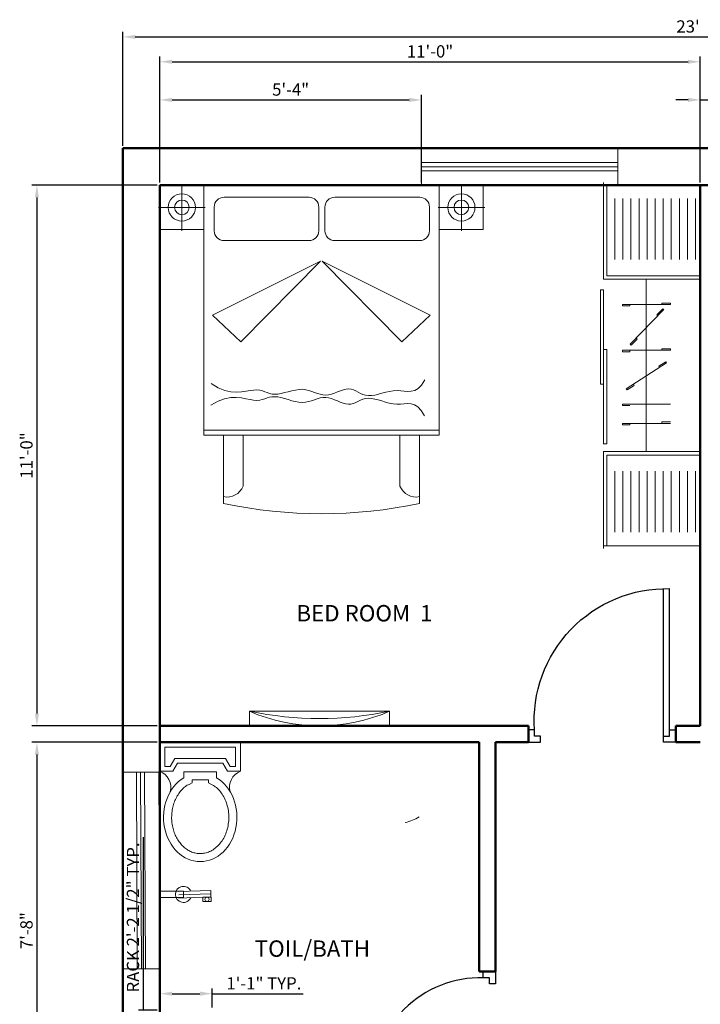
# Model space of a CAD drawing. Units: inches. Extents: x 108 to 1546, y -229 to 513.
# Tile 2 of 11: x 108 to 274, y 147 to 388. Entities that reach past the tile are written whole.
import ezdxf

# ---------------------------------------------------------------- set-up
doc = ezdxf.new("R2010")
doc.units = ezdxf.units.IN
for name, color, linetype, lineweight in [('A-ANNO-DIMS', 2, 'Continuous', 18), ('A-AREA-IDEN', 4, 'Continuous', 18), ('A-FLOR-FIXT', 9, 'Continuous', 18), ('A-FURN', 8, 'Continuous', 13), ('door', 1, 'Continuous', 25), ('tv', 2, 'Continuous', 13), ('wall', 7, 'Continuous', 50), ('WINDOW', 212, 'Continuous', 18)]:
    doc.layers.add(name, color=color, linetype=linetype, lineweight=lineweight)
doc.styles.get("Standard").update_dxf_attribs({"font": 'arial.ttf'})
doc.dimstyles.new('ISO-25', dxfattribs={"dimtxt": 3, "dimasz": 3, "dimexe": 1.25, "dimexo": 0.625, "dimtad": 1, "dimdec": 1, "dimlunit": 3, "dimtxsty": 'Standard', "dimcen": 2.5, "dimadec": 0, "dimazin": 0, "dimtfac": 1, "dimtdec": 1, "dimtmove": 0, "dimatfit": 3, "dimfxl": 1, "dimarcsym": 0})

# ---------------------------------------------------------------- blocks, each defined once
blk = doc.blocks.new('A$C4F543DC7')
for p, q in [((0.013, 3.35, -0.169), (3.313, 3.35, -0.169)), ((0.463, 3.35, -0.169), (0.013, 3.35, -0.169)), ((0.013, 2.896, -0.169), (0.013, 3.35, -0.169)), ((0.013, 3.35, -0.169), (0.013, 2.896, -0.169)), ((0.238, 3.123, -0.439), (0.238, 3.361, -0.439)), ((0.463, 3.35, -0.169), (0.463, 0.8, -0.169)), ((2.863, 3.35, -0.169), (0.463, 3.35, -0.169)), ((0.463, 2.896, -0.169), (0.463, 3.35, -0.169)), ((2.863, 0.8, -0.169), (2.863, 3.35, -0.169)), ((2.863, 3.35, -0.169), (3.313, 3.35, -0.169)), ((2.863, 2.896, -0.169), (2.863, 3.35, -0.169)), ((3.089, 3.123, -0.439), (3.089, 3.361, -0.439)), ((3.313, 3.35, -0.169), (3.313, 2.896, -0.169)), ((3.313, 3.35, -0.169), (3.313, 2.896, -0.169)), ((1.535, 3.226, -0.169), (0.668, 3.226, -0.169)), ((2.664, 3.226, -0.169), (1.797, 3.226, -0.169)), ((0.238, 3.123, -0.439), (0, 3.123, -0.439)), ((0.238, 3.123, -0.439), (0.476, 3.123, -0.439)), ((0.238, 3.123, -0.439), (0.238, 2.885, -0.439)), ((0.568, 3.126, -0.169), (0.568, 2.884, -0.169)), ((1.635, 2.884, -0.169), (1.635, 3.126, -0.169)), ((1.697, 3.126, -0.169), (1.697, 2.884, -0.169)), ((2.764, 2.884, -0.169), (2.764, 3.126, -0.169)), ((3.089, 3.123, -0.439), (2.851, 3.123, -0.439)), ((3.089, 3.123, -0.439), (3.089, 2.885, -0.439)), ((3.089, 3.123, -0.439), (3.327, 3.123, -0.439)), ((0.463, 2.896, -0.169), (0.013, 2.896, -0.169)), ((0.013, 2.896, -0.169), (0.463, 2.896, -0.169)), ((0.463, 0.8, -0.169), (0.463, 2.896, -0.169)), ((2.863, 2.896, -0.169), (2.863, 0.8, -0.169)), ((3.313, 2.896, -0.169), (2.863, 2.896, -0.169)), ((3.313, 2.896, -0.169), (2.863, 2.896, -0.169)), ((0.668, 2.784, -0.169), (1.535, 2.784, -0.169)), ((1.797, 2.784, -0.169), (2.664, 2.784, -0.169)), ((1.653, 2.573, -0.169), (0.55, 2.025, -0.169)), ((0.841, 1.752, -0.169), (1.653, 2.573, -0.169)), ((2.481, 1.752, -0.169), (1.669, 2.573, -0.169)), ((1.669, 2.573, -0.169), (2.772, 2.025, -0.169)), ((0.55, 2.025, -0.169), (0.841, 1.752, -0.169)), ((2.772, 2.025, -0.169), (2.481, 1.752, -0.169)), ((0.537, 1.327, -0.169), (0.609, 1.284, -0.169)), ((2.648, 1.277, -0.169), (2.683, 1.312, -0.169)), ((2.683, 1.312, -0.169), (2.718, 1.364, -0.169)), ((0.609, 1.284, -0.169), (0.676, 1.257, -0.169)), ((0.676, 1.257, -0.169), (0.737, 1.243, -0.169)), ((0.737, 1.243, -0.169), (0.794, 1.239, -0.169)), ((0.794, 1.239, -0.169), (0.846, 1.242, -0.169)), ((0.846, 1.242, -0.169), (0.893, 1.249, -0.169)), ((0.893, 1.249, -0.169), (0.935, 1.256, -0.169)), ((0.935, 1.256, -0.169), (0.972, 1.261, -0.169)), ((0.972, 1.261, -0.169), (1.004, 1.262, -0.169)), ((1.004, 1.262, -0.169), (1.033, 1.258, -0.169)), ((1.033, 1.258, -0.169), (1.06, 1.251, -0.169)), ((1.06, 1.251, -0.169), (1.084, 1.242, -0.169)), ((1.084, 1.242, -0.169), (1.108, 1.234, -0.169)), ((1.108, 1.234, -0.169), (1.132, 1.226, -0.169)), ((1.132, 1.226, -0.169), (1.158, 1.22, -0.169)), ((1.158, 1.22, -0.169), (1.185, 1.218, -0.169)), ((1.185, 1.218, -0.169), (1.216, 1.22, -0.169)), ((1.216, 1.22, -0.169), (1.25, 1.226, -0.169)), ((1.25, 1.226, -0.169), (1.285, 1.235, -0.169)), ((1.285, 1.235, -0.169), (1.322, 1.244, -0.169)), ((1.322, 1.244, -0.169), (1.359, 1.253, -0.169)), ((1.359, 1.253, -0.169), (1.396, 1.261, -0.169)), ((1.396, 1.261, -0.169), (1.433, 1.266, -0.169)), ((1.433, 1.266, -0.169), (1.468, 1.268, -0.169)), ((1.468, 1.268, -0.169), (1.501, 1.264, -0.169)), ((1.501, 1.264, -0.169), (1.532, 1.257, -0.169)), ((1.532, 1.257, -0.169), (1.562, 1.247, -0.169)), ((1.562, 1.247, -0.169), (1.591, 1.237, -0.169)), ((1.591, 1.237, -0.169), (1.62, 1.226, -0.169)), ((1.62, 1.226, -0.169), (1.648, 1.217, -0.169)), ((1.648, 1.217, -0.169), (1.676, 1.211, -0.169)), ((1.676, 1.211, -0.169), (1.705, 1.209, -0.169)), ((1.705, 1.209, -0.169), (1.735, 1.212, -0.169)), ((1.735, 1.212, -0.169), (1.765, 1.22, -0.169)), ((1.765, 1.22, -0.169), (1.795, 1.23, -0.169)), ((1.795, 1.23, -0.169), (1.826, 1.242, -0.169)), ((1.826, 1.242, -0.169), (1.856, 1.253, -0.169)), ((1.856, 1.253, -0.169), (1.885, 1.263, -0.169)), ((1.885, 1.263, -0.169), (1.913, 1.27, -0.169)), ((1.913, 1.27, -0.169), (1.94, 1.272, -0.169)), ((1.94, 1.272, -0.169), (1.965, 1.269, -0.169)), ((1.965, 1.269, -0.169), (1.989, 1.262, -0.169)), ((1.989, 1.262, -0.169), (2.012, 1.251, -0.169)), ((2.012, 1.251, -0.169), (2.036, 1.239, -0.169)), ((2.036, 1.239, -0.169), (2.06, 1.227, -0.169)), ((2.06, 1.227, -0.169), (2.085, 1.216, -0.169)), ((2.085, 1.216, -0.169), (2.112, 1.208, -0.169)), ((2.112, 1.208, -0.169), (2.141, 1.204, -0.169)), ((2.141, 1.204, -0.169), (2.172, 1.205, -0.169)), ((2.172, 1.205, -0.169), (2.206, 1.21, -0.169)), ((2.206, 1.21, -0.169), (2.242, 1.218, -0.169)), ((2.242, 1.218, -0.169), (2.279, 1.228, -0.169)), ((2.279, 1.228, -0.169), (2.317, 1.238, -0.169)), ((2.317, 1.238, -0.169), (2.356, 1.246, -0.169)), ((2.356, 1.246, -0.169), (2.394, 1.253, -0.169)), ((2.394, 1.253, -0.169), (2.433, 1.255, -0.169)), ((2.433, 1.255, -0.169), (2.47, 1.253, -0.169)), ((2.47, 1.253, -0.169), (2.506, 1.249, -0.169)), ((2.506, 1.249, -0.169), (2.542, 1.246, -0.169)), ((2.542, 1.246, -0.169), (2.578, 1.248, -0.169)), ((2.578, 1.248, -0.169), (2.613, 1.257, -0.169)), ((2.613, 1.257, -0.169), (2.648, 1.277, -0.169)), ((0.533, 1.105, -0.169), (0.607, 1.146, -0.169)), ((0.607, 1.146, -0.169), (0.674, 1.171, -0.169)), ((0.674, 1.171, -0.169), (0.736, 1.183, -0.169)), ((0.736, 1.183, -0.169), (0.793, 1.185, -0.169)), ((0.793, 1.185, -0.169), (0.845, 1.18, -0.169)), ((0.845, 1.18, -0.169), (0.891, 1.172, -0.169)), ((0.891, 1.172, -0.169), (0.933, 1.163, -0.169)), ((0.933, 1.163, -0.169), (0.97, 1.156, -0.169)), ((0.97, 1.156, -0.169), (1.003, 1.155, -0.169)), ((1.003, 1.155, -0.169), (1.032, 1.158, -0.169)), ((1.032, 1.158, -0.169), (1.058, 1.164, -0.169)), ((1.058, 1.164, -0.169), (1.083, 1.172, -0.169)), ((1.083, 1.172, -0.169), (1.107, 1.18, -0.169)), ((1.107, 1.18, -0.169), (1.132, 1.187, -0.169)), ((1.132, 1.187, -0.169), (1.157, 1.192, -0.169)), ((1.157, 1.192, -0.169), (1.185, 1.193, -0.169)), ((1.185, 1.193, -0.169), (1.216, 1.19, -0.169)), ((1.216, 1.19, -0.169), (1.249, 1.183, -0.169)), ((1.249, 1.183, -0.169), (1.284, 1.173, -0.169)), ((1.284, 1.173, -0.169), (1.321, 1.163, -0.169)), ((1.321, 1.163, -0.169), (1.358, 1.152, -0.169)), ((1.358, 1.152, -0.169), (1.394, 1.143, -0.169)), ((1.394, 1.143, -0.169), (1.431, 1.137, -0.169)), ((1.431, 1.137, -0.169), (1.466, 1.135, -0.169)), ((1.466, 1.135, -0.169), (1.499, 1.137, -0.169)), ((1.499, 1.137, -0.169), (1.531, 1.143, -0.169)), ((1.531, 1.143, -0.169), (1.561, 1.152, -0.169)), ((1.561, 1.152, -0.169), (1.59, 1.162, -0.169)), ((1.59, 1.162, -0.169), (1.619, 1.172, -0.169)), ((1.619, 1.172, -0.169), (1.648, 1.18, -0.169)), ((1.648, 1.18, -0.169), (1.676, 1.185, -0.169)), ((1.676, 1.185, -0.169), (1.705, 1.186, -0.169)), ((1.705, 1.186, -0.169), (1.734, 1.182, -0.169)), ((1.734, 1.182, -0.169), (1.764, 1.173, -0.169)), ((1.764, 1.173, -0.169), (1.794, 1.162, -0.169)), ((1.794, 1.162, -0.169), (1.824, 1.149, -0.169)), ((1.824, 1.149, -0.169), (1.854, 1.137, -0.169)), ((1.854, 1.137, -0.169), (1.883, 1.126, -0.169)), ((1.883, 1.126, -0.169), (1.911, 1.119, -0.169)), ((1.911, 1.119, -0.169), (1.937, 1.115, -0.169)), ((1.937, 1.115, -0.169), (1.963, 1.118, -0.169)), ((1.963, 1.118, -0.169), (1.987, 1.124, -0.169)), ((1.987, 1.124, -0.169), (2.011, 1.134, -0.169)), ((2.011, 1.134, -0.169), (2.034, 1.145, -0.169)), ((2.034, 1.145, -0.169), (2.059, 1.157, -0.169)), ((2.059, 1.157, -0.169), (2.084, 1.167, -0.169)), ((2.084, 1.167, -0.169), (2.111, 1.174, -0.169)), ((2.111, 1.174, -0.169), (2.14, 1.177, -0.169)), ((2.14, 1.177, -0.169), (2.172, 1.175, -0.169)), ((2.172, 1.175, -0.169), (2.206, 1.169, -0.169)), ((2.206, 1.169, -0.169), (2.241, 1.16, -0.169)), ((2.241, 1.16, -0.169), (2.278, 1.149, -0.169)), ((2.278, 1.149, -0.169), (2.316, 1.138, -0.169)), ((2.316, 1.138, -0.169), (2.354, 1.128, -0.169)), ((2.354, 1.128, -0.169), (2.392, 1.121, -0.169)), ((2.392, 1.121, -0.169), (2.43, 1.117, -0.169)), ((2.43, 1.117, -0.169), (2.468, 1.118, -0.169)), ((2.468, 1.118, -0.169), (2.504, 1.121, -0.169)), ((2.504, 1.121, -0.169), (2.54, 1.123, -0.169)), ((2.54, 1.123, -0.169), (2.576, 1.12, -0.169)), ((2.576, 1.12, -0.169), (2.611, 1.109, -0.169)), ((2.611, 1.109, -0.169), (2.645, 1.088, -0.169)), ((2.645, 1.088, -0.169), (2.679, 1.052, -0.169)), ((2.679, 1.052, -0.169), (2.712, 0.999, -0.169)), ((0.463, 0.85, -0.169), (2.863, 0.85, -0.169)), ((0.463, 0.8, -0.169), (2.863, 0.8, -0.169)), ((0.663, 0.8, -0.169), (0.463, 0.8, -0.169)), ((0.663, 0.8, -0.169), (2.663, 0.8, -0.169)), ((0.663, 0.104, -0.169), (0.663, 0.8, -0.169)), ((0.663, 0.104, -0.169), (0.663, 0.8, -0.169)), ((0.863, 0.281, -0.169), (0.863, 0.8, -0.169)), ((2.463, 0.8, -0.169), (2.463, 0.281, -0.169)), ((2.863, 0.8, -0.169), (2.663, 0.8, -0.169)), ((2.663, 0.8, -0.169), (2.663, 0.104, -0.169)), ((2.663, 0.8, -0.169), (2.663, 0.104, -0.169))]:
    blk.add_line(p, q)
for centre, radius in [((0.238, 3.123, -0.439), 0.139), ((3.089, 3.123, -0.439), 0.139), ((0.238, 3.123, -0.439), 0.075), ((3.089, 3.123, -0.439), 0.075)]:
    blk.add_circle(centre, radius)
for centre, radius, start, end in [((0.668, 3.126, -0.169), 0.1, 90, 180), ((1.535, 3.126, -0.169), 0.1, 0, 90), ((1.797, 3.126, -0.169), 0.1, 90, 180), ((2.664, 3.126, -0.169), 0.1, 0, 90), ((0.668, 2.884, -0.169), 0.1, 180, 270), ((1.535, 2.884, -0.169), 0.1, 270, 0), ((1.797, 2.884, -0.169), 0.1, 180, 270), ((2.664, 2.884, -0.169), 0.1, 270, 0), ((0.699, 0.347, -0.169), 0.177, 258.2616, 338.032), ((2.627, 0.347, -0.169), 0.177, 201.968, 281.7384), ((1.663, 4.86, -0.169), 4.86, 258.1252, 281.8748), ((1.663, 4.86, -0.169), 4.86, 258.1252, 281.8748)]:
    blk.add_arc(centre, radius, start, end)
blk = doc.blocks.new('A$C34930FF8')
for p, q in [((600, 1669.3), (600, 2269.3)), ((580, 1690.9), (580, 2252.4)), ((30, 1790.9), (30, 2169.3)), ((80, 1790.9), (80, 2169.3)), ((130, 1790.9), (130, 2169.3)), ((180, 1790.9), (180, 2169.3)), ((230, 1790.9), (230, 2169.3)), ((280, 1790.9), (280, 2169.3)), ((330, 1790.9), (330, 2169.3)), ((380, 1790.9), (380, 2169.3)), ((430, 1790.9), (430, 2169.3)), ((480, 1790.9), (480, 2169.3)), ((530, 1790.9), (530, 2169.3)), ((580, 1690.9), (0, 1690.9)), ((600, 1669.3), (0, 1669.3)), ((335.4, 1666.1), (335.4, 603.1)), ((600, 1603.3), (620, 1603.3)), ((600, 1018.7), (600, 1603.3)), ((620, 1603.3), (620, 1018.7)), ((237.7, 1521.5), (185.4, 1521.5)), ((482.5, 1513), (185.4, 1513)), ((434.8, 1266.1), (227.4, 1478.9)), ((269.7, 1447.7), (233.2, 1485.2)), ((436.7, 1504.4), (482.5, 1504.4)), ((428.7, 1260.1), (392.1, 1297.6)), ((237.7, 1237.7), (185.4, 1237.7)), ((482.5, 1228.2), (185.4, 1228.2)), ((600, 1233.4), (580, 1233.4)), ((580, 1233.4), (580, 648.7)), ((600, 648.7), (600, 1233.4)), ((436.7, 1219.7), (482.5, 1219.7)), ((459.3, 989.3), (209.5, 1150.1)), ((258.1, 1129), (214.1, 1157.3)), ((454.7, 982.1), (410.6, 1010.5)), ((620, 1018.7), (600, 1018.7)), ((482.5, 894.9), (185.4, 894.9)), ((436.7, 886.3), (482.5, 886.3)), ((237.7, 783.9), (185.4, 783.9)), ((482.5, 775.3), (185.4, 775.3)), ((436.7, 766.8), (482.5, 766.8)), ((580, 648.7), (600, 648.7)), ((600, 600), (0, 600)), ((580, 578.3), (0, 578.3)), ((580, 578.3), (580, 16.8)), ((600, 600), (600, 0)), ((30, 478.3), (30, 100)), ((80, 478.3), (80, 100)), ((130, 478.3), (130, 100)), ((180, 478.3), (180, 100)), ((230, 478.3), (230, 100)), ((280, 478.3), (280, 100)), ((330, 478.3), (330, 100)), ((380, 478.3), (380, 100)), ((430, 478.3), (430, 100)), ((480, 478.3), (480, 100)), ((530, 478.3), (530, 100))]:
    blk.add_line(p, q)
at = {"ltscale": 0.05}
for p, q in [((0, 2252.4), (0, 16.8)), ((600, 2252.4), (0, 2252.4)), ((185.4, 1513), (185.4, 1521.5)), ((227.1, 1479.2), (233.2, 1485.2)), ((237.7, 1513), (237.7, 1521.5)), ((436.7, 1513), (436.7, 1504.4)), ((482.5, 1513), (482.5, 1504.4)), ((263.6, 1441.7), (269.7, 1447.7)), ((398.2, 1303.6), (392.1, 1297.6)), ((185.4, 1229.1), (185.4, 1237.7)), ((237.7, 1229.1), (237.7, 1237.7)), ((434.8, 1266.1), (428.7, 1260.1)), ((436.7, 1228.2), (436.7, 1219.7)), ((482.5, 1228.2), (482.5, 1219.7)), ((209.5, 1150.1), (214.1, 1157.3)), ((253.5, 1121.8), (258.1, 1129)), ((415.3, 1017.6), (410.6, 1010.5)), ((459.3, 989.3), (454.7, 982.1)), ((482.5, 894.9), (482.5, 886.3)), ((237.7, 775.3), (237.7, 783.9)), ((436.7, 775.3), (436.7, 766.8)), ((482.5, 775.3), (482.5, 766.8)), ((600, 16.8), (0, 16.8))]:
    blk.add_line(p, q, dxfattribs=at)
blk = doc.blocks.new('A$C7C8779AE')
for p, q in [((0, 0.7405), (0, 0.5605)), ((0.5, 0.7405), (0, 0.7405)), ((0.5, 0.5605), (0.5, 0.7405)), ((0.47, 0.7105), (0.03, 0.7105)), ((0.03, 0.7105), (0.03, 0.5905)), ((0.47, 0.5905), (0.47, 0.7105)), ((0.093, 0.6405), (0.063, 0.5905)), ((0.093, 0.6405), (0.407, 0.6405)), ((0.437, 0.5905), (0.407, 0.6405)), ((0, 0.5605), (0.08, 0.5605)), ((0.03, 0.5905), (0.063, 0.5905)), ((0.11, 0.6105), (0.08, 0.5605)), ((0.11, 0.6105), (0.39, 0.6105)), ((0.1497, 0.557), (0.1497, 0.5203)), ((0.1497, 0.557), (0.3514, 0.557)), ((0.3514, 0.557), (0.3514, 0.5203)), ((0.42, 0.5605), (0.39, 0.6105)), ((0.42, 0.5605), (0.5, 0.5605)), ((0.437, 0.5905), (0.47, 0.5905)), ((0.1997, 0.507), (0.1997, 0.4879)), ((0.1997, 0.507), (0.3014, 0.507)), ((0.3014, 0.507), (0.3014, 0.4879))]:
    blk.add_line(p, q)
for centre, start, end in [((-0.0386, 0.4613), 344.64203, 68.73386), ((0.5386, 0.4613), 111.26614, 195.35797)]:
    blk.add_arc(centre, 0.1064, start, end)
blk.add_ellipse((0.2506, 0.2744), major_axis=(0, 0.2744), ratio=0.828948, start_param=0.459479, end_param=5.823706)
blk.add_open_spline([(0.1997, 0.4879), (0.1697, 0.474), (0.1642, 0.4702), (0.1512, 0.4602), (0.1438, 0.4535), (0.1298, 0.4388), (0.1233, 0.4306), (0.1111, 0.4131), (0.1055, 0.4037), (0.0956, 0.3838), (0.0912, 0.3733), (0.0838, 0.3516), (0.0808, 0.3403), (0.0762, 0.3172), (0.0746, 0.3055), (0.073, 0.2817), (0.0729, 0.2698), (0.0743, 0.246), (0.0758, 0.2342), (0.0801, 0.2111), (0.0831, 0.1998), (0.0903, 0.1779), (0.0945, 0.1673), (0.1043, 0.1473), (0.1098, 0.1378), (0.1218, 0.12), (0.1283, 0.1118), (0.1421, 0.0968), (0.1494, 0.09), (0.1646, 0.078), (0.1725, 0.0728), (0.1887, 0.064), (0.1969, 0.0603), (0.2137, 0.0547), (0.2222, 0.0527), (0.2392, 0.0502), (0.2478, 0.0498), (0.2664, 0.0505), (0.2764, 0.052), (0.2963, 0.0573), (0.3061, 0.061), (0.3253, 0.0707), (0.3346, 0.0766), (0.3525, 0.0906), (0.3611, 0.0987), (0.3771, 0.1169), (0.3845, 0.127), (0.3978, 0.1488), (0.4037, 0.1605), (0.4137, 0.1853), (0.4178, 0.1983), (0.424, 0.2251), (0.4261, 0.2389), (0.4282, 0.2668), (0.4283, 0.2809), (0.4262, 0.3088), (0.4241, 0.3226), (0.418, 0.3495), (0.414, 0.3625), (0.404, 0.3873), (0.3982, 0.3991), (0.385, 0.421), (0.3776, 0.4311), (0.3617, 0.4494), (0.3531, 0.4575), (0.3382, 0.4693), (0.3321, 0.4736), (0.3014, 0.4879)], degree=3, knots=[0.459479, 0.459479, 0.459479, 0.459479, 0.567422, 0.567422, 0.720865, 0.720865, 0.874307, 0.874307, 1.02775, 1.02775, 1.181192, 1.181192, 1.334635, 1.334635, 1.488077, 1.488077, 1.64152, 1.64152, 1.794963, 1.794963, 1.948405, 1.948405, 2.101848, 2.101848, 2.25529, 2.25529, 2.408733, 2.408733, 2.562175, 2.562175, 2.715618, 2.715618, 2.86906, 2.86906, 3.022503, 3.022503, 3.175946, 3.175946, 3.356457, 3.356457, 3.536968, 3.536968, 3.717479, 3.717479, 3.89799, 3.89799, 4.078501, 4.078501, 4.259012, 4.259012, 4.439523, 4.439523, 4.620035, 4.620035, 4.800546, 4.800546, 4.981057, 4.981057, 5.161568, 5.161568, 5.342079, 5.342079, 5.52259, 5.52259, 5.703101, 5.703101, 5.823706, 5.823706, 5.823706, 5.823706])
blk = doc.blocks.new('*D21')
at = {"layer": 'A-ANNO-DIMS', "color": 0, "lineweight": -2, "transparency": 16777216}
for p, q in [((132.92, 357.09), (132.92, 384.9)), ((408.92, 357.09), (408.92, 384.9)), ((135.92, 383.65), (405.92, 383.65))]:
    blk.add_line(p, q, dxfattribs=at)
at = {"layer": 'A-ANNO-DIMS', "color": 0, "transparency": 16777216}
for points in [[(135.92, 384.15), (135.92, 383.15), (132.92, 383.65)], [(405.92, 384.15), (405.92, 383.15), (408.92, 383.65)]]:
    blk.add_solid(points, dxfattribs=at)
at = {"layer": 'Defpoints', "color": 0, "transparency": 16777216}
for p in [(408.92, 383.65), (132.92, 356.47), (408.92, 356.47)]:
    blk.add_point(p, dxfattribs=at)
at = {"layer": 'A-ANNO-DIMS', "color": 0, "transparency": 16777216, "insert": (270.92, 385.81), "char_height": 3, "attachment_point": 5}
blk.add_mtext("23'", dxfattribs=at)
blk = doc.blocks.new('WINDOW-48X9')
for p, q in [((0, 9), (0, 0)), ((0, 9), (48, 9)), ((48, 9), (48, 0)), ((0, 5.5), (48, 5.5)), ((0, 4.5), (48, 4.5)), ((0, 3.5), (48, 3.5)), ((0, 0), (48, 0))]:
    blk.add_line(p, q)
blk = doc.blocks.new('DOOR-SWING-36')
for p, q in [((1.5, 1.5), (1.5, 37.5)), ((3, 1.5), (3, 37.5)), ((0, 3), (0, 0)), ((1.5, 3), (0, 3)), ((1.5, 1.5), (1.5, 3)), ((34.5, 1.5), (34.5, 3)), ((34.5, 3), (36, 3)), ((36, 3), (36, 0)), ((3, 1.5), (1.5, 1.5)), ((3, 0), (3, 1.5)), ((33, 0), (33, 1.5)), ((33, 1.5), (34.5, 1.5)), ((0, 0), (3, 0)), ((36, 0), (33, 0))]:
    blk.add_line(p, q)
blk.add_arc((2.25, 5.18), 32.32, 356.1244, 91.3295)
blk = doc.blocks.new('DOOR-SWING-30')
for p, q in [((27, 30), (30, 30)), ((27, 28.5), (27, 30)), ((30, 30), (30, 27)), ((28.5, 28.5), (27, 28.5)), ((28.5, 27), (28.5, 28.5)), ((30, 27), (28.5, 27)), ((30, 3), (0, 3)), ((30, 3), (28.5, 3)), ((28.5, 3), (28.5, 1.5)), ((30, 0), (30, 3)), ((28.5, 1.5), (0, 1.5)), ((28.5, 1.5), (27, 1.5)), ((27, 1.5), (27, 0)), ((27, 0), (30, 0))]:
    blk.add_line(p, q)
blk.add_arc((26.25, 2.25), 26.26, 88.3634, 181.6366)
blk = doc.blocks.new('TV-WALL-MOUNT')
blk.add_lwpolyline([(0, 0), (34.19, 0), (34.19, 3.56), (0, 3.56)], close=True)
for centre, radius, start, end in [((17.1, 42.8), 42.8, 246.4582, 293.5418), ((17.1, 84.72), 82.93, 258.1036, 281.8964)]:
    blk.add_arc(centre, radius, start, end)
blk = doc.blocks.new('*D68')
at = {"layer": 'A-ANNO-DIMS', "color": 0, "lineweight": -2, "transparency": 16777216}
for p, q in [((137.93, 146.1), (137.93, 188.28)), ((141.3, 146.1), (136.68, 146.1)), ((137.93, 122.47), (137.93, 143.1)), ((141.3, 119.47), (136.68, 119.47))]:
    blk.add_line(p, q, dxfattribs=at)
at = {"layer": 'A-ANNO-DIMS', "color": 0, "transparency": 16777216}
for points in [[(137.43, 143.1), (138.43, 143.1), (137.93, 146.1)], [(137.43, 122.47), (138.43, 122.47), (137.93, 119.47)]]:
    blk.add_solid(points, dxfattribs=at)
at = {"layer": 'Defpoints', "color": 0, "transparency": 16777216}
for p in [(137.93, 146.1), (141.92, 146.1), (141.92, 119.47)]:
    blk.add_point(p, dxfattribs=at)
at = {"layer": 'A-ANNO-DIMS', "color": 0, "transparency": 16777216, "insert": (135.75, 168.69), "char_height": 3, "attachment_point": 5, "rotation": 90}
blk.add_mtext('RACK 2\'-2 1/2" TYP.', dxfattribs=at)
blk = doc.blocks.new('*D69')
at = {"layer": 'A-ANNO-DIMS', "color": 0, "lineweight": -2, "transparency": 16777216}
for p, q in [((141.92, 146.72), (141.92, 151.34)), ((144.92, 150.09), (151.7, 150.09)), ((154.7, 146.72), (154.7, 151.34)), ((154.7, 150.09), (176.96, 150.09))]:
    blk.add_line(p, q, dxfattribs=at)
at = {"layer": 'A-ANNO-DIMS', "color": 0, "transparency": 16777216}
for points in [[(144.92, 150.59), (144.92, 149.59), (141.92, 150.09)], [(151.7, 150.59), (151.7, 149.59), (154.7, 150.09)]]:
    blk.add_solid(points, dxfattribs=at)
at = {"layer": 'Defpoints', "color": 0, "transparency": 16777216}
for p in [(154.7, 150.09), (141.92, 146.1), (154.7, 146.1)]:
    blk.add_point(p, dxfattribs=at)
at = {"layer": 'A-ANNO-DIMS', "color": 0, "transparency": 16777216, "insert": (167.33, 152.22), "char_height": 3, "attachment_point": 5}
blk.add_mtext('1\'-1" TYP.', dxfattribs=at)
blk = doc.blocks.new('*D72')
at = {"layer": 'A-ANNO-DIMS', "color": 0, "lineweight": -2, "transparency": 16777216}
for p, q in [((141.92, 348.09), (141.92, 378.83)), ((144.92, 377.58), (270.92, 377.58)), ((273.92, 348.09), (273.92, 378.83))]:
    blk.add_line(p, q, dxfattribs=at)
at = {"layer": 'A-ANNO-DIMS', "color": 0, "transparency": 16777216}
for points in [[(144.92, 378.08), (144.92, 377.08), (141.92, 377.58)], [(270.92, 378.08), (270.92, 377.08), (273.92, 377.58)]]:
    blk.add_solid(points, dxfattribs=at)
at = {"layer": 'Defpoints', "color": 0, "transparency": 16777216}
for p in [(273.92, 377.58), (141.92, 347.47), (273.92, 347.47)]:
    blk.add_point(p, dxfattribs=at)
at = {"layer": 'A-ANNO-DIMS', "color": 0, "transparency": 16777216, "insert": (207.92, 379.73), "char_height": 3, "attachment_point": 5}
blk.add_mtext('11\'-0"', dxfattribs=at)
blk = doc.blocks.new('*D76')
at = {"layer": 'A-ANNO-DIMS', "color": 0, "lineweight": -2, "transparency": 16777216}
for p, q in [((141.3, 347.47), (110.64, 347.47)), ((111.89, 344.47), (111.89, 218.47)), ((141.3, 215.47), (110.64, 215.47))]:
    blk.add_line(p, q, dxfattribs=at)
at = {"layer": 'A-ANNO-DIMS', "color": 0, "transparency": 16777216}
for points in [[(111.39, 344.47), (112.39, 344.47), (111.89, 347.47)], [(111.39, 218.47), (112.39, 218.47), (111.89, 215.47)]]:
    blk.add_solid(points, dxfattribs=at)
at = {"layer": 'Defpoints', "color": 0, "transparency": 16777216}
for p in [(141.92, 347.47), (111.89, 215.47), (141.92, 215.47)]:
    blk.add_point(p, dxfattribs=at)
at = {"layer": 'A-ANNO-DIMS', "color": 0, "transparency": 16777216, "insert": (109.73, 281.47), "char_height": 3, "attachment_point": 5, "rotation": 90}
blk.add_mtext('11\'-0"', dxfattribs=at)
blk = doc.blocks.new('*D77')
at = {"layer": 'A-ANNO-DIMS', "color": 0, "lineweight": -2, "transparency": 16777216}
for p, q in [((141.3, 211.47), (110.64, 211.47)), ((111.89, 208.47), (111.89, 122.47)), ((141.3, 119.47), (110.64, 119.47))]:
    blk.add_line(p, q, dxfattribs=at)
at = {"layer": 'A-ANNO-DIMS', "color": 0, "transparency": 16777216}
for points in [[(111.39, 208.47), (112.39, 208.47), (111.89, 211.47)], [(111.39, 122.47), (112.39, 122.47), (111.89, 119.47)]]:
    blk.add_solid(points, dxfattribs=at)
at = {"layer": 'Defpoints', "color": 0, "transparency": 16777216}
for p in [(141.92, 211.47), (111.89, 119.47), (141.92, 119.47)]:
    blk.add_point(p, dxfattribs=at)
at = {"layer": 'A-ANNO-DIMS', "color": 0, "transparency": 16777216, "insert": (109.73, 165.47), "char_height": 3, "attachment_point": 5, "rotation": 90}
blk.add_mtext('7\'-8"', dxfattribs=at)
blk = doc.blocks.new('*D80')
at = {"layer": 'A-ANNO-DIMS', "color": 0, "lineweight": -2, "transparency": 16777216}
for p, q in [((270.92, 368.27), (267.92, 368.27)), ((273.92, 348.09), (273.92, 369.52)), ((273.92, 368.27), (277.92, 368.27)), ((277.92, 348.09), (277.92, 369.52)), ((280.92, 368.27), (293.15, 368.27))]:
    blk.add_line(p, q, dxfattribs=at)
at = {"layer": 'A-ANNO-DIMS', "color": 0, "transparency": 16777216}
for points in [[(270.92, 368.77), (270.92, 367.77), (273.92, 368.27)], [(280.92, 368.77), (280.92, 367.77), (277.92, 368.27)]]:
    blk.add_solid(points, dxfattribs=at)
at = {"layer": 'Defpoints', "color": 0, "transparency": 16777216}
for p in [(277.92, 368.27), (273.92, 347.47), (277.92, 347.47)]:
    blk.add_point(p, dxfattribs=at)
at = {"layer": 'A-ANNO-DIMS', "color": 0, "transparency": 16777216, "insert": (288.53, 370.43), "char_height": 3, "attachment_point": 5}
blk.add_mtext('0\'-4"', dxfattribs=at)
blk = doc.blocks.new('*D81')
at = {"layer": 'A-ANNO-DIMS', "color": 0, "lineweight": -2, "transparency": 16777216}
for p, q in [((141.92, 348.09), (141.92, 369.52)), ((144.92, 368.27), (202.8, 368.27)), ((205.8, 348.09), (205.8, 369.52))]:
    blk.add_line(p, q, dxfattribs=at)
at = {"layer": 'A-ANNO-DIMS', "color": 0, "transparency": 16777216}
for points in [[(144.92, 368.77), (144.92, 367.77), (141.92, 368.27)], [(202.8, 368.77), (202.8, 367.77), (205.8, 368.27)]]:
    blk.add_solid(points, dxfattribs=at)
at = {"layer": 'Defpoints', "color": 0, "transparency": 16777216}
for p in [(205.8, 368.27), (141.92, 347.47), (205.8, 347.47)]:
    blk.add_point(p, dxfattribs=at)
at = {"layer": 'A-ANNO-DIMS', "color": 0, "transparency": 16777216, "insert": (173.86, 370.42), "char_height": 3, "attachment_point": 5}
blk.add_mtext('5\'-4"', dxfattribs=at)

msp = doc.modelspace()

# ---------------------------------------------------------------- linework, layer by layer
at = {"layer": 'A-FLOR-FIXT'}
for p, q in [((146.49, 175.01), (154.36, 175.26)), ((146.52, 174.22), (154.39, 174.47)), ((146.54, 173.44), (154.41, 173.69)), ((154.41, 173.69), (154.36, 175.26))]:
    msp.add_line(p, q, dxfattribs=at)
for points in [[(141.92, 175.1), (147.68, 175.1), (147.68, 173.55), (141.92, 173.55)], [(152.4, 173.62), (154.46, 173.62), (154.46, 172.59), (152.4, 172.59)]]:
    msp.add_lwpolyline(points, close=True, dxfattribs=at)
msp.add_circle((153.43, 173.11), 0.517, dxfattribs=at)
for centre, radius, start, end in [((198.88, 204.31), 12.8, 283.4853, 300.0686), ((147.68, 174.32), 1.96, 23.5435, 336.034)]:
    msp.add_arc(centre, radius, start, end, dxfattribs=at)
at = {"layer": 'wall'}
for p, q in [((408.92, 356.47), (132.92, 356.47)), ((132.92, 356.47), (132.92, -3.53)), ((399.92, 347.47), (141.92, 347.47)), ((141.92, 347.47), (141.92, 5.47)), ((273.92, 347.47), (273.92, 215.47)), ((231.92, 215.47), (141.92, 215.47)), ((231.92, 215.47), (231.92, 211.47)), ((273.92, 215.47), (267.92, 215.47)), ((267.92, 215.47), (267.92, 211.47)), ((219.92, 211.47), (141.92, 211.47)), ((219.92, 211.47), (219.92, 155.47)), ((223.92, 211.47), (223.92, 155.47)), ((231.92, 211.47), (223.92, 211.47)), ((273.92, 211.47), (267.92, 211.47)), ((219.92, 155.47), (223.92, 155.47))]:
    msp.add_line(p, q, dxfattribs=at)

# ---------------------------------------------------------------- block references
at = {"layer": 'A-FLOR-FIXT', "xscale": 39.37007874015748, "yscale": 39.37007874015748, "zscale": 39.37007874015748}
msp.add_blockref('A$C7C8779AE', (141.92, 182.32), dxfattribs=at)
at = {"layer": 'A-FURN', "xscale": 23.94379789781286, "yscale": 23.94379789781286, "zscale": 23.94379789781286}
msp.add_blockref('A$C4F543DC7', (141.6, 267.26, 4.04), dxfattribs=at)
at = {"layer": 'A-FURN', "xscale": -0.0393700787401575, "yscale": 0.0393700787401575, "zscale": 0.0393700787401575, "rotation": 359.9999999999957}
msp.add_blockref('A$C34930FF8', (273.92, 258.79), dxfattribs=at)
at = {"layer": 'door', "extrusion": (0, 0, -1), "zscale": -1}
msp.add_blockref('DOOR-SWING-36', (-267.92, 211.47), dxfattribs=at)
at = {"layer": 'door'}
msp.add_blockref('DOOR-SWING-30', (193.92, 125.47), dxfattribs=at)
at = {"layer": 'tv'}
msp.add_blockref('TV-WALL-MOUNT', (163.82, 215.47), dxfattribs=at)
at = {"layer": 'WINDOW'}
msp.add_blockref('WINDOW-48X9', (205.8, 347.47), dxfattribs=at)
at = {"layer": 'WINDOW', "rotation": 90.2799560098106}
msp.add_blockref('WINDOW-48X9', (141.92, 156.19), dxfattribs=at)

# ---------------------------------------------------------------- texts
at = {"layer": 'A-AREA-IDEN', "char_height": 4, "attachment_point": 1}
for s, insert in [('BED ROOM  1', (175.27, 244.96)), ('TOIL/BATH', (165.1, 163.09))]:
    msp.add_mtext_dynamic_manual_height_columns(s, width=57.4311, gutter_width=12.5, heights=[12.84], dxfattribs=dict(at, insert=insert))

# ---------------------------------------------------------------- dimensions: what is measured, and where the dimension line sits
at = {"layer": 'A-ANNO-DIMS'}
for base, p1, p2, override, picture, middle in [((408.92, 383.65), (132.92, 356.47), (408.92, 356.47), {"dimclrd": 0, "dimclre": 0, "dimclrt": 0}, '*D21', (270.92, 385.81)), ((273.92, 377.58), (141.92, 347.47), (273.92, 347.47), {"dimdec": 1, "dimlfac": 1, "dimrnd": 0, "dimzin": 1, "dimdsep": 46, "dimlunit": 4, "dimfrac": 2}, '*D72', (207.92, 379.73)), ((277.92, 368.27), (273.92, 347.47), (277.92, 347.47), {"dimdec": 1, "dimlfac": 1, "dimrnd": 0, "dimzin": 1, "dimdsep": 46, "dimlunit": 4, "dimfrac": 2}, '*D80', (288.53, 370.43))]:
    dim = msp.add_linear_dim(base=base, p1=p1, p2=p2, dimstyle='ISO-25', override=override, dxfattribs=at)
    dim.commit()
    dim.dimension.update_dxf_attribs({"geometry": picture, "text_midpoint": middle})
for base, p1, p2, angle, picture, middle in [((205.8, 368.27), (141.92, 347.47), (205.8, 347.47), 0, '*D81', (173.86, 370.42)), ((111.89, 215.47), (141.92, 347.47), (141.92, 215.47), 90, '*D76', (109.73, 281.47)), ((111.89, 119.47), (141.92, 211.47), (141.92, 119.47), 90, '*D77', (109.73, 165.47))]:
    dim = msp.add_linear_dim(base=base, p1=p1, p2=p2, angle=angle, dimstyle='ISO-25', override={"dimdec": 1, "dimlfac": 1, "dimrnd": 0, "dimzin": 1, "dimdsep": 46, "dimlunit": 4, "dimfrac": 2}, dxfattribs=at)
    dim.commit()
    dim.dimension.update_dxf_attribs({"geometry": picture, "text_midpoint": middle})
dim = msp.add_linear_dim(base=(137.93, 146.1), p1=(141.92, 119.47), p2=(141.92, 146.1), angle=90, text='RACK <> TYP.', dimstyle='ISO-25', override={"dimdec": 1, "dimlfac": 1, "dimrnd": 0, "dimzin": 1, "dimdsep": 46, "dimlunit": 4, "dimfrac": 2}, dxfattribs=at)
dim.commit()
dim.dimension.update_dxf_attribs({"geometry": '*D68', "text_midpoint": (135.75, 168.69)})
dim = msp.add_linear_dim(base=(154.7, 150.09), p1=(141.92, 146.1), p2=(154.7, 146.1), text='<> TYP.', dimstyle='ISO-25', override={"dimdec": 1, "dimlfac": 1, "dimrnd": 0, "dimzin": 1, "dimdsep": 46, "dimlunit": 4, "dimfrac": 2}, dxfattribs=at)
dim.commit()
dim.dimension.update_dxf_attribs({"geometry": '*D69', "text_midpoint": (167.33, 152.22)})

doc.saveas('drawing.dxf')
